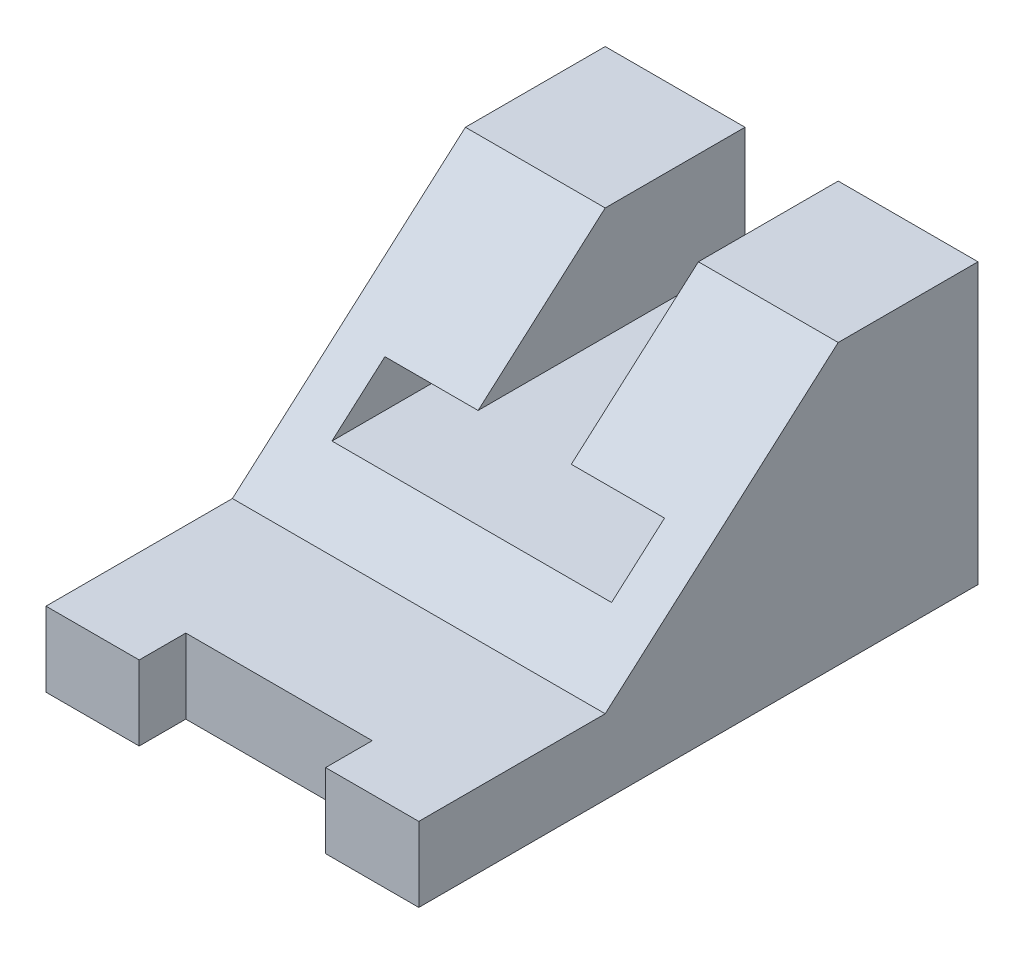
ISO-10303-21;
HEADER;
FILE_DESCRIPTION(('STEP AP214'),'2;1');
FILE_NAME('part.step','',(''),(''),'','','');
FILE_SCHEMA(('AUTOMOTIVE_DESIGN { 1 0 10303 214 1 1 1 1 }'));
ENDSEC;
DATA;
#1=APPLICATION_CONTEXT('core data for automotive mechanical design processes');
#2=APPLICATION_PROTOCOL_DEFINITION('international standard','automotive_design',2000,#1);
#3=PRODUCT_CONTEXT('',#1,'mechanical');
#4=PRODUCT('Part','Part','',(#3));
#5=PRODUCT_RELATED_PRODUCT_CATEGORY('part','',(#4));
#6=PRODUCT_DEFINITION_FORMATION('','',#4);
#7=PRODUCT_DEFINITION_CONTEXT('part definition',#1,'design');
#8=PRODUCT_DEFINITION('design','',#6,#7);
#9=PRODUCT_DEFINITION_SHAPE('','',#8);
#10=(LENGTH_UNIT() NAMED_UNIT(*) SI_UNIT(.MILLI.,.METRE.));
#11=(NAMED_UNIT(*) PLANE_ANGLE_UNIT() SI_UNIT($,.RADIAN.));
#12=(NAMED_UNIT(*) SI_UNIT($,.STERADIAN.) SOLID_ANGLE_UNIT());
#13=UNCERTAINTY_MEASURE_WITH_UNIT(LENGTH_MEASURE(1.E-05),#10,'distance_accuracy_value','');
#14=(GEOMETRIC_REPRESENTATION_CONTEXT(3) GLOBAL_UNCERTAINTY_ASSIGNED_CONTEXT((#13)) GLOBAL_UNIT_ASSIGNED_CONTEXT((#10,
#11,#12)) REPRESENTATION_CONTEXT('',''));
#15=CARTESIAN_POINT('',(0.,0.,0.));
#16=DIRECTION('',(0.,0.,1.));
#17=DIRECTION('',(1.,0.,0.));
#18=AXIS2_PLACEMENT_3D('',#15,#16,#17);
#19=CARTESIAN_POINT('',(0.,8.,0.));
#20=DIRECTION('',(0.,0.,-1.));
#21=DIRECTION('',(-1.,0.,0.));
#22=AXIS2_PLACEMENT_3D('',#19,#20,#21);
#23=PLANE('',#22);
#24=DIRECTION('',(1.,0.,0.));
#25=VECTOR('',#24,1.);
#26=CARTESIAN_POINT('',(-20.,8.,0.));
#27=LINE('',#26,#25);
#28=CARTESIAN_POINT('',(10.,8.,0.));
#29=VERTEX_POINT('',#28);
#30=CARTESIAN_POINT('',(20.,8.,0.));
#31=VERTEX_POINT('',#30);
#32=EDGE_CURVE('E263',#29,#31,#27,.T.);
#33=ORIENTED_EDGE('',*,*,#32,.F.);
#34=DIRECTION('',(0.,1.,0.));
#35=VECTOR('',#34,1.);
#36=CARTESIAN_POINT('',(10.,-32.,0.));
#37=LINE('',#36,#35);
#38=CARTESIAN_POINT('',(10.,0.,0.));
#39=VERTEX_POINT('',#38);
#40=EDGE_CURVE('E198',#39,#29,#37,.T.);
#41=ORIENTED_EDGE('',*,*,#40,.F.);
#42=DIRECTION('',(1.,0.,0.));
#43=VECTOR('',#42,1.);
#44=CARTESIAN_POINT('',(0.,0.,0.));
#45=LINE('',#44,#43);
#46=CARTESIAN_POINT('',(20.,0.,0.));
#47=VERTEX_POINT('',#46);
#48=EDGE_CURVE('E258',#39,#47,#45,.T.);
#49=ORIENTED_EDGE('',*,*,#48,.T.);
#50=DIRECTION('',(0.,-1.,0.));
#51=VECTOR('',#50,1.);
#52=CARTESIAN_POINT('',(20.,8.,0.));
#53=LINE('',#52,#51);
#54=EDGE_CURVE('E290',#31,#47,#53,.T.);
#55=ORIENTED_EDGE('',*,*,#54,.F.);
#56=EDGE_LOOP('',(#33,#41,#49,#55));
#57=FACE_BOUND('',#56,.T.);
#58=ADVANCED_FACE('F44',(#57),#23,.F.);
#59=CARTESIAN_POINT('',(0.,8.,0.));
#60=DIRECTION('',(0.,1.,0.));
#61=DIRECTION('',(0.,0.,1.));
#62=AXIS2_PLACEMENT_3D('',#59,#60,#61);
#63=PLANE('',#62);
#64=DIRECTION('',(0.,0.,-1.));
#65=VECTOR('',#64,1.);
#66=CARTESIAN_POINT('',(10.,8.,-5.));
#67=LINE('',#66,#65);
#68=CARTESIAN_POINT('',(10.,8.,-5.));
#69=VERTEX_POINT('',#68);
#70=EDGE_CURVE('E183',#29,#69,#67,.T.);
#71=ORIENTED_EDGE('',*,*,#70,.F.);
#72=ORIENTED_EDGE('',*,*,#32,.T.);
#73=DIRECTION('',(0.,0.,-1.));
#74=VECTOR('',#73,1.);
#75=CARTESIAN_POINT('',(20.,8.,0.));
#76=LINE('',#75,#74);
#77=CARTESIAN_POINT('',(20.,7.99999999999999,-20.));
#78=VERTEX_POINT('',#77);
#79=EDGE_CURVE('E265',#31,#78,#76,.T.);
#80=ORIENTED_EDGE('',*,*,#79,.T.);
#81=DIRECTION('',(1.,0.,0.));
#82=VECTOR('',#81,1.);
#83=CARTESIAN_POINT('',(5.,7.99999999999999,-20.));
#84=LINE('',#83,#82);
#85=CARTESIAN_POINT('',(-20.,7.99999999999999,-20.));
#86=VERTEX_POINT('',#85);
#87=EDGE_CURVE('E255',#86,#78,#84,.T.);
#88=ORIENTED_EDGE('',*,*,#87,.F.);
#89=DIRECTION('',(0.,0.,1.));
#90=VECTOR('',#89,1.);
#91=CARTESIAN_POINT('',(-20.,8.,-60.));
#92=LINE('',#91,#90);
#93=CARTESIAN_POINT('',(-20.,8.,0.));
#94=VERTEX_POINT('',#93);
#95=EDGE_CURVE('E266',#86,#94,#92,.T.);
#96=ORIENTED_EDGE('',*,*,#95,.T.);
#97=CARTESIAN_POINT('',(-10.,8.,0.));
#98=VERTEX_POINT('',#97);
#99=EDGE_CURVE('E186',#94,#98,#27,.T.);
#100=ORIENTED_EDGE('',*,*,#99,.T.);
#101=DIRECTION('',(0.,0.,1.));
#102=VECTOR('',#101,1.);
#103=CARTESIAN_POINT('',(-10.,8.,0.));
#104=LINE('',#103,#102);
#105=CARTESIAN_POINT('',(-10.,8.,-5.));
#106=VERTEX_POINT('',#105);
#107=EDGE_CURVE('E175',#106,#98,#104,.T.);
#108=ORIENTED_EDGE('',*,*,#107,.F.);
#109=DIRECTION('',(-1.,0.,0.));
#110=VECTOR('',#109,1.);
#111=CARTESIAN_POINT('',(0.,8.,-5.));
#112=LINE('',#111,#110);
#113=EDGE_CURVE('E177',#69,#106,#112,.T.);
#114=ORIENTED_EDGE('',*,*,#113,.F.);
#115=EDGE_LOOP('',(#71,#72,#80,#88,#96,#100,#108,#114));
#116=FACE_BOUND('',#115,.T.);
#117=ADVANCED_FACE('F188',(#116),#63,.T.);
#118=CARTESIAN_POINT('',(5.,0.,0.));
#119=DIRECTION('',(-1.,0.,0.));
#120=DIRECTION('',(0.,0.,1.));
#121=AXIS2_PLACEMENT_3D('',#118,#119,#120);
#122=PLANE('',#121);
#123=DIRECTION('',(0.,1.,0.));
#124=VECTOR('',#123,1.);
#125=CARTESIAN_POINT('',(5.,8.,-60.));
#126=LINE('',#125,#124);
#127=CARTESIAN_POINT('',(5.,18.,-60.));
#128=VERTEX_POINT('',#127);
#129=CARTESIAN_POINT('',(5.,30.,-60.));
#130=VERTEX_POINT('',#129);
#131=EDGE_CURVE('E238',#128,#130,#126,.T.);
#132=ORIENTED_EDGE('',*,*,#131,.F.);
#133=DIRECTION('',(0.,0.,-1.));
#134=VECTOR('',#133,1.);
#135=CARTESIAN_POINT('',(5.,18.,-60.));
#136=LINE('',#135,#134);
#137=CARTESIAN_POINT('',(5.,18.,-31.3636363636364));
#138=VERTEX_POINT('',#137);
#139=EDGE_CURVE('E217',#138,#128,#136,.T.);
#140=ORIENTED_EDGE('',*,*,#139,.F.);
#141=DIRECTION('',(0.,-0.660627894892025,0.750713516922755));
#142=VECTOR('',#141,1.);
#143=CARTESIAN_POINT('',(5.,7.99999999999999,-20.));
#144=LINE('',#143,#142);
#145=CARTESIAN_POINT('',(5.,30.,-45.));
#146=VERTEX_POINT('',#145);
#147=EDGE_CURVE('E247',#146,#138,#144,.T.);
#148=ORIENTED_EDGE('',*,*,#147,.F.);
#149=DIRECTION('',(0.,0.,1.));
#150=VECTOR('',#149,1.);
#151=CARTESIAN_POINT('',(5.,30.,-60.));
#152=LINE('',#151,#150);
#153=EDGE_CURVE('E245',#130,#146,#152,.T.);
#154=ORIENTED_EDGE('',*,*,#153,.F.);
#155=EDGE_LOOP('',(#132,#140,#148,#154));
#156=FACE_BOUND('',#155,.T.);
#157=ADVANCED_FACE('F339',(#156),#122,.T.);
#158=CARTESIAN_POINT('',(-5.,0.,0.));
#159=DIRECTION('',(1.,0.,0.));
#160=DIRECTION('',(0.,0.,-1.));
#161=AXIS2_PLACEMENT_3D('',#158,#159,#160);
#162=PLANE('',#161);
#163=DIRECTION('',(0.,0.660627894892025,-0.750713516922755));
#164=VECTOR('',#163,1.);
#165=CARTESIAN_POINT('',(-5.,30.,-45.));
#166=LINE('',#165,#164);
#167=CARTESIAN_POINT('',(-5.,18.,-31.3636363636364));
#168=VERTEX_POINT('',#167);
#169=CARTESIAN_POINT('',(-5.,30.,-45.));
#170=VERTEX_POINT('',#169);
#171=EDGE_CURVE('E222',#168,#170,#166,.T.);
#172=ORIENTED_EDGE('',*,*,#171,.F.);
#173=DIRECTION('',(0.,0.,1.));
#174=VECTOR('',#173,1.);
#175=CARTESIAN_POINT('',(-5.,18.,-20.));
#176=LINE('',#175,#174);
#177=CARTESIAN_POINT('',(-5.,18.,-60.));
#178=VERTEX_POINT('',#177);
#179=EDGE_CURVE('E211',#178,#168,#176,.T.);
#180=ORIENTED_EDGE('',*,*,#179,.F.);
#181=DIRECTION('',(0.,-1.,0.));
#182=VECTOR('',#181,1.);
#183=CARTESIAN_POINT('',(-5.,8.,-60.));
#184=LINE('',#183,#182);
#185=CARTESIAN_POINT('',(-5.,30.,-60.));
#186=VERTEX_POINT('',#185);
#187=EDGE_CURVE('E230',#186,#178,#184,.T.);
#188=ORIENTED_EDGE('',*,*,#187,.F.);
#189=DIRECTION('',(0.,0.,-1.));
#190=VECTOR('',#189,1.);
#191=CARTESIAN_POINT('',(-5.,30.,-60.));
#192=LINE('',#191,#190);
#193=EDGE_CURVE('E224',#170,#186,#192,.T.);
#194=ORIENTED_EDGE('',*,*,#193,.F.);
#195=EDGE_LOOP('',(#172,#180,#188,#194));
#196=FACE_BOUND('',#195,.T.);
#197=ADVANCED_FACE('F334',(#196),#162,.T.);
#198=CARTESIAN_POINT('',(-20.,0.,0.));
#199=VERTEX_POINT('',#198);
#200=CARTESIAN_POINT('',(-10.,0.,0.));
#201=VERTEX_POINT('',#200);
#202=EDGE_CURVE('E267',#199,#201,#45,.T.);
#203=ORIENTED_EDGE('',*,*,#202,.T.);
#204=DIRECTION('',(0.,1.,0.));
#205=VECTOR('',#204,1.);
#206=CARTESIAN_POINT('',(-10.,-32.,0.));
#207=LINE('',#206,#205);
#208=EDGE_CURVE('E58',#201,#98,#207,.T.);
#209=ORIENTED_EDGE('',*,*,#208,.T.);
#210=ORIENTED_EDGE('',*,*,#99,.F.);
#211=DIRECTION('',(0.,-1.,0.));
#212=VECTOR('',#211,1.);
#213=CARTESIAN_POINT('',(-20.,8.,0.));
#214=LINE('',#213,#212);
#215=EDGE_CURVE('E268',#94,#199,#214,.T.);
#216=ORIENTED_EDGE('',*,*,#215,.T.);
#217=EDGE_LOOP('',(#203,#209,#210,#216));
#218=FACE_BOUND('',#217,.T.);
#219=ADVANCED_FACE('F50',(#218),#23,.F.);
#220=CARTESIAN_POINT('',(20.,8.,0.));
#221=DIRECTION('',(-1.,0.,0.));
#222=DIRECTION('',(0.,0.,1.));
#223=AXIS2_PLACEMENT_3D('',#220,#221,#222);
#224=PLANE('',#223);
#225=DIRECTION('',(0.,0.,-1.));
#226=VECTOR('',#225,1.);
#227=CARTESIAN_POINT('',(20.,0.,0.));
#228=LINE('',#227,#226);
#229=CARTESIAN_POINT('',(20.,0.,-60.));
#230=VERTEX_POINT('',#229);
#231=EDGE_CURVE('E275',#47,#230,#228,.T.);
#232=ORIENTED_EDGE('',*,*,#231,.T.);
#233=DIRECTION('',(0.,-1.,0.));
#234=VECTOR('',#233,1.);
#235=CARTESIAN_POINT('',(20.,8.,-60.));
#236=LINE('',#235,#234);
#237=CARTESIAN_POINT('',(20.,30.,-60.));
#238=VERTEX_POINT('',#237);
#239=EDGE_CURVE('E284',#238,#230,#236,.T.);
#240=ORIENTED_EDGE('',*,*,#239,.F.);
#241=DIRECTION('',(0.,0.,1.));
#242=VECTOR('',#241,1.);
#243=CARTESIAN_POINT('',(20.,30.,-60.));
#244=LINE('',#243,#242);
#245=CARTESIAN_POINT('',(20.,30.,-45.));
#246=VERTEX_POINT('',#245);
#247=EDGE_CURVE('E240',#238,#246,#244,.T.);
#248=ORIENTED_EDGE('',*,*,#247,.T.);
#249=DIRECTION('',(0.,-0.660627894892025,0.750713516922755));
#250=VECTOR('',#249,1.);
#251=CARTESIAN_POINT('',(20.,7.99999999999999,-20.));
#252=LINE('',#251,#250);
#253=EDGE_CURVE('E243',#246,#78,#252,.T.);
#254=ORIENTED_EDGE('',*,*,#253,.T.);
#255=ORIENTED_EDGE('',*,*,#79,.F.);
#256=ORIENTED_EDGE('',*,*,#54,.T.);
#257=EDGE_LOOP('',(#232,#240,#248,#254,#255,#256));
#258=FACE_BOUND('',#257,.T.);
#259=ADVANCED_FACE('F313',(#258),#224,.F.);
#260=CARTESIAN_POINT('',(20.,8.,-60.));
#261=DIRECTION('',(0.,0.,1.));
#262=DIRECTION('',(1.,0.,0.));
#263=AXIS2_PLACEMENT_3D('',#260,#261,#262);
#264=PLANE('',#263);
#265=DIRECTION('',(0.,-1.,0.));
#266=VECTOR('',#265,1.);
#267=CARTESIAN_POINT('',(15.,18.,-60.));
#268=LINE('',#267,#266);
#269=CARTESIAN_POINT('',(15.,18.,-60.));
#270=VERTEX_POINT('',#269);
#271=CARTESIAN_POINT('',(15.,13.,-60.));
#272=VERTEX_POINT('',#271);
#273=EDGE_CURVE('E206',#270,#272,#268,.T.);
#274=ORIENTED_EDGE('',*,*,#273,.F.);
#275=DIRECTION('',(1.,0.,0.));
#276=VECTOR('',#275,1.);
#277=CARTESIAN_POINT('',(-15.,18.,-60.));
#278=LINE('',#277,#276);
#279=EDGE_CURVE('E201',#128,#270,#278,.T.);
#280=ORIENTED_EDGE('',*,*,#279,.F.);
#281=ORIENTED_EDGE('',*,*,#131,.T.);
#282=DIRECTION('',(1.,0.,0.));
#283=VECTOR('',#282,1.);
#284=CARTESIAN_POINT('',(5.,30.,-60.));
#285=LINE('',#284,#283);
#286=EDGE_CURVE('E246',#130,#238,#285,.T.);
#287=ORIENTED_EDGE('',*,*,#286,.T.);
#288=ORIENTED_EDGE('',*,*,#239,.T.);
#289=DIRECTION('',(-1.,0.,0.));
#290=VECTOR('',#289,1.);
#291=CARTESIAN_POINT('',(20.,0.,-60.));
#292=LINE('',#291,#290);
#293=CARTESIAN_POINT('',(-20.,0.,-60.));
#294=VERTEX_POINT('',#293);
#295=EDGE_CURVE('E273',#230,#294,#292,.T.);
#296=ORIENTED_EDGE('',*,*,#295,.T.);
#297=DIRECTION('',(0.,-1.,0.));
#298=VECTOR('',#297,1.);
#299=CARTESIAN_POINT('',(-20.,8.,-60.));
#300=LINE('',#299,#298);
#301=CARTESIAN_POINT('',(-20.,30.,-60.));
#302=VERTEX_POINT('',#301);
#303=EDGE_CURVE('E282',#302,#294,#300,.T.);
#304=ORIENTED_EDGE('',*,*,#303,.F.);
#305=DIRECTION('',(-1.,0.,0.));
#306=VECTOR('',#305,1.);
#307=CARTESIAN_POINT('',(-5.,30.,-60.));
#308=LINE('',#307,#306);
#309=EDGE_CURVE('E231',#186,#302,#308,.T.);
#310=ORIENTED_EDGE('',*,*,#309,.F.);
#311=ORIENTED_EDGE('',*,*,#187,.T.);
#312=CARTESIAN_POINT('',(-15.,18.,-60.));
#313=VERTEX_POINT('',#312);
#314=EDGE_CURVE('E204',#313,#178,#278,.T.);
#315=ORIENTED_EDGE('',*,*,#314,.F.);
#316=DIRECTION('',(0.,1.,0.));
#317=VECTOR('',#316,1.);
#318=CARTESIAN_POINT('',(-15.,13.,-60.));
#319=LINE('',#318,#317);
#320=CARTESIAN_POINT('',(-15.,13.,-60.));
#321=VERTEX_POINT('',#320);
#322=EDGE_CURVE('E199',#321,#313,#319,.T.);
#323=ORIENTED_EDGE('',*,*,#322,.F.);
#324=DIRECTION('',(-1.,0.,0.));
#325=VECTOR('',#324,1.);
#326=CARTESIAN_POINT('',(0.,13.,-60.));
#327=LINE('',#326,#325);
#328=EDGE_CURVE('E193',#272,#321,#327,.T.);
#329=ORIENTED_EDGE('',*,*,#328,.F.);
#330=EDGE_LOOP('',(#274,#280,#281,#287,#288,#296,#304,#310,#311,#315,#323,#329));
#331=FACE_BOUND('',#330,.T.);
#332=ADVANCED_FACE('F338',(#331),#264,.F.);
#333=CARTESIAN_POINT('',(-20.,8.,-60.));
#334=DIRECTION('',(1.,0.,0.));
#335=DIRECTION('',(0.,0.,-1.));
#336=AXIS2_PLACEMENT_3D('',#333,#334,#335);
#337=PLANE('',#336);
#338=DIRECTION('',(0.,0.,1.));
#339=VECTOR('',#338,1.);
#340=CARTESIAN_POINT('',(-20.,0.,-60.));
#341=LINE('',#340,#339);
#342=EDGE_CURVE('E277',#294,#199,#341,.T.);
#343=ORIENTED_EDGE('',*,*,#342,.T.);
#344=ORIENTED_EDGE('',*,*,#215,.F.);
#345=ORIENTED_EDGE('',*,*,#95,.F.);
#346=DIRECTION('',(0.,0.660627894892025,-0.750713516922755));
#347=VECTOR('',#346,1.);
#348=CARTESIAN_POINT('',(-20.,30.,-45.));
#349=LINE('',#348,#347);
#350=CARTESIAN_POINT('',(-20.,30.,-45.));
#351=VERTEX_POINT('',#350);
#352=EDGE_CURVE('E219',#86,#351,#349,.T.);
#353=ORIENTED_EDGE('',*,*,#352,.T.);
#354=DIRECTION('',(0.,0.,-1.));
#355=VECTOR('',#354,1.);
#356=CARTESIAN_POINT('',(-20.,30.,-60.));
#357=LINE('',#356,#355);
#358=EDGE_CURVE('E221',#351,#302,#357,.T.);
#359=ORIENTED_EDGE('',*,*,#358,.T.);
#360=ORIENTED_EDGE('',*,*,#303,.T.);
#361=EDGE_LOOP('',(#343,#344,#345,#353,#359,#360));
#362=FACE_BOUND('',#361,.T.);
#363=ADVANCED_FACE('F318',(#362),#337,.F.);
#364=CARTESIAN_POINT('',(0.,0.,0.));
#365=DIRECTION('',(0.,1.,0.));
#366=DIRECTION('',(0.,0.,1.));
#367=AXIS2_PLACEMENT_3D('',#364,#365,#366);
#368=PLANE('',#367);
#369=ORIENTED_EDGE('',*,*,#48,.F.);
#370=DIRECTION('',(0.,0.,-1.));
#371=VECTOR('',#370,1.);
#372=CARTESIAN_POINT('',(10.,0.,0.));
#373=LINE('',#372,#371);
#374=CARTESIAN_POINT('',(10.,0.,-5.));
#375=VERTEX_POINT('',#374);
#376=EDGE_CURVE('E11',#39,#375,#373,.T.);
#377=ORIENTED_EDGE('',*,*,#376,.T.);
#378=DIRECTION('',(-1.,0.,0.));
#379=VECTOR('',#378,1.);
#380=CARTESIAN_POINT('',(0.,0.,-5.));
#381=LINE('',#380,#379);
#382=CARTESIAN_POINT('',(-10.,0.,-5.));
#383=VERTEX_POINT('',#382);
#384=EDGE_CURVE('E52',#375,#383,#381,.T.);
#385=ORIENTED_EDGE('',*,*,#384,.T.);
#386=DIRECTION('',(0.,0.,1.));
#387=VECTOR('',#386,1.);
#388=CARTESIAN_POINT('',(-10.,0.,0.));
#389=LINE('',#388,#387);
#390=EDGE_CURVE('E173',#383,#201,#389,.T.);
#391=ORIENTED_EDGE('',*,*,#390,.T.);
#392=ORIENTED_EDGE('',*,*,#202,.F.);
#393=ORIENTED_EDGE('',*,*,#342,.F.);
#394=ORIENTED_EDGE('',*,*,#295,.F.);
#395=ORIENTED_EDGE('',*,*,#231,.F.);
#396=EDGE_LOOP('',(#369,#377,#385,#391,#392,#393,#394,#395));
#397=FACE_BOUND('',#396,.T.);
#398=ADVANCED_FACE('F302',(#397),#368,.F.);
#399=CARTESIAN_POINT('',(5.,7.99999999999999,-20.));
#400=DIRECTION('',(0.,0.750713516922755,0.660627894892025));
#401=DIRECTION('',(0.,-0.660627894892025,0.750713516922755));
#402=AXIS2_PLACEMENT_3D('',#399,#400,#401);
#403=PLANE('',#402);
#404=DIRECTION('',(-1.,0.,0.));
#405=VECTOR('',#404,1.);
#406=CARTESIAN_POINT('',(5.,18.,-31.3636363636364));
#407=LINE('',#406,#405);
#408=CARTESIAN_POINT('',(15.,18.,-31.3636363636364));
#409=VERTEX_POINT('',#408);
#410=EDGE_CURVE('E300',#409,#138,#407,.T.);
#411=ORIENTED_EDGE('',*,*,#410,.F.);
#412=DIRECTION('',(0.,0.660627894892025,-0.750713516922755));
#413=VECTOR('',#412,1.);
#414=CARTESIAN_POINT('',(15.,7.99999999999999,-20.));
#415=LINE('',#414,#413);
#416=CARTESIAN_POINT('',(15.,13.,-25.6818181818182));
#417=VERTEX_POINT('',#416);
#418=EDGE_CURVE('E297',#417,#409,#415,.T.);
#419=ORIENTED_EDGE('',*,*,#418,.F.);
#420=DIRECTION('',(1.,0.,0.));
#421=VECTOR('',#420,1.);
#422=CARTESIAN_POINT('',(5.,13.,-25.6818181818182));
#423=LINE('',#422,#421);
#424=CARTESIAN_POINT('',(-15.,13.,-25.6818181818182));
#425=VERTEX_POINT('',#424);
#426=EDGE_CURVE('E288',#425,#417,#423,.T.);
#427=ORIENTED_EDGE('',*,*,#426,.F.);
#428=DIRECTION('',(0.,-0.660627894892025,0.750713516922755));
#429=VECTOR('',#428,1.);
#430=CARTESIAN_POINT('',(-15.,7.99999999999999,-20.));
#431=LINE('',#430,#429);
#432=CARTESIAN_POINT('',(-15.,18.,-31.3636363636364));
#433=VERTEX_POINT('',#432);
#434=EDGE_CURVE('E295',#433,#425,#431,.T.);
#435=ORIENTED_EDGE('',*,*,#434,.F.);
#436=EDGE_CURVE('E294',#168,#433,#407,.T.);
#437=ORIENTED_EDGE('',*,*,#436,.F.);
#438=ORIENTED_EDGE('',*,*,#171,.T.);
#439=DIRECTION('',(-1.,0.,0.));
#440=VECTOR('',#439,1.);
#441=CARTESIAN_POINT('',(-5.,30.,-45.));
#442=LINE('',#441,#440);
#443=EDGE_CURVE('E226',#170,#351,#442,.T.);
#444=ORIENTED_EDGE('',*,*,#443,.T.);
#445=ORIENTED_EDGE('',*,*,#352,.F.);
#446=ORIENTED_EDGE('',*,*,#87,.T.);
#447=ORIENTED_EDGE('',*,*,#253,.F.);
#448=DIRECTION('',(1.,0.,0.));
#449=VECTOR('',#448,1.);
#450=CARTESIAN_POINT('',(5.,30.,-45.));
#451=LINE('',#450,#449);
#452=EDGE_CURVE('E260',#146,#246,#451,.T.);
#453=ORIENTED_EDGE('',*,*,#452,.F.);
#454=ORIENTED_EDGE('',*,*,#147,.T.);
#455=EDGE_LOOP('',(#411,#419,#427,#435,#437,#438,#444,#445,#446,#447,#453,#454));
#456=FACE_BOUND('',#455,.T.);
#457=ADVANCED_FACE('F319',(#456),#403,.T.);
#458=CARTESIAN_POINT('',(5.,30.,-60.));
#459=DIRECTION('',(0.,1.,0.));
#460=DIRECTION('',(0.,0.,1.));
#461=AXIS2_PLACEMENT_3D('',#458,#459,#460);
#462=PLANE('',#461);
#463=ORIENTED_EDGE('',*,*,#247,.F.);
#464=ORIENTED_EDGE('',*,*,#286,.F.);
#465=ORIENTED_EDGE('',*,*,#153,.T.);
#466=ORIENTED_EDGE('',*,*,#452,.T.);
#467=EDGE_LOOP('',(#463,#464,#465,#466));
#468=FACE_BOUND('',#467,.T.);
#469=ADVANCED_FACE('F354',(#468),#462,.T.);
#470=CARTESIAN_POINT('',(-5.,30.,-60.));
#471=DIRECTION('',(0.,1.,0.));
#472=DIRECTION('',(0.,0.,1.));
#473=AXIS2_PLACEMENT_3D('',#470,#471,#472);
#474=PLANE('',#473);
#475=ORIENTED_EDGE('',*,*,#358,.F.);
#476=ORIENTED_EDGE('',*,*,#443,.F.);
#477=ORIENTED_EDGE('',*,*,#193,.T.);
#478=ORIENTED_EDGE('',*,*,#309,.T.);
#479=EDGE_LOOP('',(#475,#476,#477,#478));
#480=FACE_BOUND('',#479,.T.);
#481=ADVANCED_FACE('F330',(#480),#474,.T.);
#482=CARTESIAN_POINT('',(-15.,18.,-20.));
#483=DIRECTION('',(0.,1.,0.));
#484=DIRECTION('',(-1.,0.,0.));
#485=AXIS2_PLACEMENT_3D('',#482,#483,#484);
#486=PLANE('',#485);
#487=ORIENTED_EDGE('',*,*,#139,.T.);
#488=ORIENTED_EDGE('',*,*,#279,.T.);
#489=DIRECTION('',(0.,0.,-1.));
#490=VECTOR('',#489,1.);
#491=CARTESIAN_POINT('',(15.,18.,-20.));
#492=LINE('',#491,#490);
#493=EDGE_CURVE('E215',#409,#270,#492,.T.);
#494=ORIENTED_EDGE('',*,*,#493,.F.);
#495=ORIENTED_EDGE('',*,*,#410,.T.);
#496=EDGE_LOOP('',(#487,#488,#494,#495));
#497=FACE_BOUND('',#496,.T.);
#498=ADVANCED_FACE('F374',(#497),#486,.F.);
#499=CARTESIAN_POINT('',(15.,18.,-20.));
#500=DIRECTION('',(1.,0.,0.));
#501=DIRECTION('',(0.,0.,-1.));
#502=AXIS2_PLACEMENT_3D('',#499,#500,#501);
#503=PLANE('',#502);
#504=ORIENTED_EDGE('',*,*,#418,.T.);
#505=ORIENTED_EDGE('',*,*,#493,.T.);
#506=ORIENTED_EDGE('',*,*,#273,.T.);
#507=DIRECTION('',(0.,0.,-1.));
#508=VECTOR('',#507,1.);
#509=CARTESIAN_POINT('',(15.,13.,-20.));
#510=LINE('',#509,#508);
#511=EDGE_CURVE('E207',#417,#272,#510,.T.);
#512=ORIENTED_EDGE('',*,*,#511,.F.);
#513=EDGE_LOOP('',(#504,#505,#506,#512));
#514=FACE_BOUND('',#513,.T.);
#515=ADVANCED_FACE('F371',(#514),#503,.F.);
#516=ORIENTED_EDGE('',*,*,#179,.T.);
#517=ORIENTED_EDGE('',*,*,#436,.T.);
#518=DIRECTION('',(0.,0.,-1.));
#519=VECTOR('',#518,1.);
#520=CARTESIAN_POINT('',(-15.,18.,-20.));
#521=LINE('',#520,#519);
#522=EDGE_CURVE('E212',#433,#313,#521,.T.);
#523=ORIENTED_EDGE('',*,*,#522,.T.);
#524=ORIENTED_EDGE('',*,*,#314,.T.);
#525=EDGE_LOOP('',(#516,#517,#523,#524));
#526=FACE_BOUND('',#525,.T.);
#527=ADVANCED_FACE('F400',(#526),#486,.F.);
#528=CARTESIAN_POINT('',(-15.,13.,-20.));
#529=DIRECTION('',(-1.,0.,0.));
#530=DIRECTION('',(0.,0.,1.));
#531=AXIS2_PLACEMENT_3D('',#528,#529,#530);
#532=PLANE('',#531);
#533=ORIENTED_EDGE('',*,*,#434,.T.);
#534=DIRECTION('',(0.,0.,-1.));
#535=VECTOR('',#534,1.);
#536=CARTESIAN_POINT('',(-15.,13.,-20.));
#537=LINE('',#536,#535);
#538=EDGE_CURVE('E69',#425,#321,#537,.T.);
#539=ORIENTED_EDGE('',*,*,#538,.T.);
#540=ORIENTED_EDGE('',*,*,#322,.T.);
#541=ORIENTED_EDGE('',*,*,#522,.F.);
#542=EDGE_LOOP('',(#533,#539,#540,#541));
#543=FACE_BOUND('',#542,.T.);
#544=ADVANCED_FACE('F394',(#543),#532,.F.);
#545=CARTESIAN_POINT('',(0.,13.,-20.));
#546=DIRECTION('',(0.,-1.,0.));
#547=DIRECTION('',(0.,0.,-1.));
#548=AXIS2_PLACEMENT_3D('',#545,#546,#547);
#549=PLANE('',#548);
#550=ORIENTED_EDGE('',*,*,#426,.T.);
#551=ORIENTED_EDGE('',*,*,#511,.T.);
#552=ORIENTED_EDGE('',*,*,#328,.T.);
#553=ORIENTED_EDGE('',*,*,#538,.F.);
#554=EDGE_LOOP('',(#550,#551,#552,#553));
#555=FACE_BOUND('',#554,.T.);
#556=ADVANCED_FACE('F392',(#555),#549,.F.);
#557=CARTESIAN_POINT('',(0.,-32.,-5.));
#558=DIRECTION('',(0.,0.,-1.));
#559=DIRECTION('',(-1.,0.,0.));
#560=AXIS2_PLACEMENT_3D('',#557,#558,#559);
#561=PLANE('',#560);
#562=DIRECTION('',(0.,1.,0.));
#563=VECTOR('',#562,1.);
#564=CARTESIAN_POINT('',(10.,-32.,-5.));
#565=LINE('',#564,#563);
#566=EDGE_CURVE('E182',#375,#69,#565,.T.);
#567=ORIENTED_EDGE('',*,*,#566,.T.);
#568=ORIENTED_EDGE('',*,*,#113,.T.);
#569=DIRECTION('',(0.,1.,0.));
#570=VECTOR('',#569,1.);
#571=CARTESIAN_POINT('',(-10.,-32.,-5.));
#572=LINE('',#571,#570);
#573=EDGE_CURVE('E169',#383,#106,#572,.T.);
#574=ORIENTED_EDGE('',*,*,#573,.F.);
#575=ORIENTED_EDGE('',*,*,#384,.F.);
#576=EDGE_LOOP('',(#567,#568,#574,#575));
#577=FACE_BOUND('',#576,.T.);
#578=ADVANCED_FACE('F176',(#577),#561,.F.);
#579=CARTESIAN_POINT('',(10.,-32.,-5.));
#580=DIRECTION('',(1.,0.,0.));
#581=DIRECTION('',(0.,0.,-1.));
#582=AXIS2_PLACEMENT_3D('',#579,#580,#581);
#583=PLANE('',#582);
#584=ORIENTED_EDGE('',*,*,#40,.T.);
#585=ORIENTED_EDGE('',*,*,#70,.T.);
#586=ORIENTED_EDGE('',*,*,#566,.F.);
#587=ORIENTED_EDGE('',*,*,#376,.F.);
#588=EDGE_LOOP('',(#584,#585,#586,#587));
#589=FACE_BOUND('',#588,.T.);
#590=ADVANCED_FACE('F304',(#589),#583,.F.);
#591=CARTESIAN_POINT('',(-10.,-32.,0.));
#592=DIRECTION('',(-1.,0.,0.));
#593=DIRECTION('',(0.,0.,1.));
#594=AXIS2_PLACEMENT_3D('',#591,#592,#593);
#595=PLANE('',#594);
#596=ORIENTED_EDGE('',*,*,#573,.T.);
#597=ORIENTED_EDGE('',*,*,#107,.T.);
#598=ORIENTED_EDGE('',*,*,#208,.F.);
#599=ORIENTED_EDGE('',*,*,#390,.F.);
#600=EDGE_LOOP('',(#596,#597,#598,#599));
#601=FACE_BOUND('',#600,.T.);
#602=ADVANCED_FACE('F168',(#601),#595,.F.);
#603=CLOSED_SHELL('',(#58,#117,#157,#197,#219,#259,#332,#363,#398,#457,#469,#481,#498,#515,#527,
#544,#556,#578,#590,#602));
#604=MANIFOLD_SOLID_BREP('B2',#603);
#605=ADVANCED_BREP_SHAPE_REPRESENTATION('',(#18,#604),#14);
#606=SHAPE_DEFINITION_REPRESENTATION(#9,#605);
ENDSEC;
END-ISO-10303-21;
